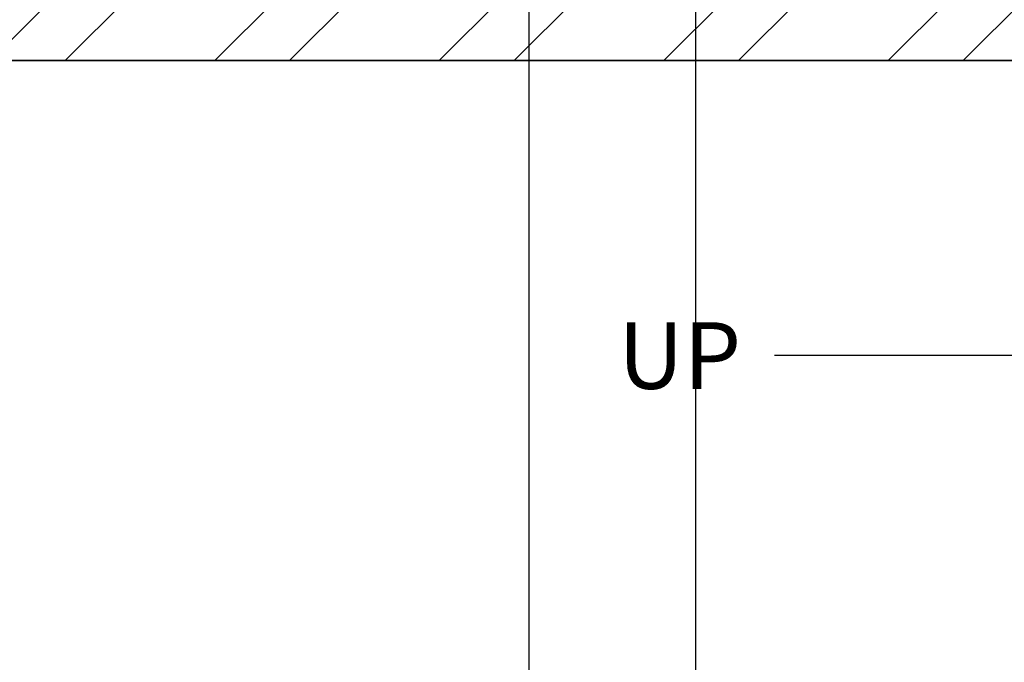
# Model space of a CAD drawing. Units: inches. Extents: x 2166 to 3588, y 1959 to 2628.
# Tile 7 of 13: x 3398 to 3457, y 2067 to 2105. Entities that reach past the tile are written whole.
import ezdxf
from ezdxf import colors
from ezdxf.entities.mleader import LeaderData, LeaderLine
from ezdxf.math import Vec2, Vec3

# ---------------------------------------------------------------- set-up
doc = ezdxf.new("R2010")
doc.units = ezdxf.units.IN
for name, color, linetype, lineweight in [('A-ANNO-DIMS', 2, 'Continuous', 18), ('A-ANNO-SYMB', 136, 'Continuous', 18), ('A-WALL-PATT', 20, 'Continuous', 13), ('WALL', 40, 'Continuous', 35)]:
    doc.layers.add(name, color=color, linetype=linetype, lineweight=lineweight)
doc.styles.get("Standard").update_dxf_attribs({"font": 'arial.ttf'})
doc.dimstyles.get("Standard").update_dxf_attribs({"dimtxt": 0.18, "dimasz": 0.18, "dimexe": 0.18, "dimexo": 0.0625, "dimgap": 0.09, "dimtad": 0, "dimtih": 1, "dimtoh": 1, "dimdec": 4, "dimzin": 0, "dimdsep": 46, "dimtxsty": 'Standard', "dimcen": 0.09, "dimadec": 0, "dimazin": 0, "dimtfac": 1, "dimtdec": 4, "dimtofl": 0, "dimtmove": 0, "dimatfit": 3, "dimfxl": 1, "dimtolj": 1, "dimtzin": 0, "dimarcsym": 0})

# ---------------------------------------------------------------- blocks, each defined once
blk = doc.blocks.new('*D53')
at = {"layer": 'A-ANNO-DIMS', "color": 0, "lineweight": -2, "transparency": 16777216}
for p, q in [((3428.471, 2066.041), (3428.471, 2454.909)), ((3428.651, 2454.729), (3433.26, 2454.729)), ((3438.291, 2454.729), (3433.681, 2454.729)), ((3438.471, 2066.041), (3438.471, 2454.909))]:
    blk.add_line(p, q, dxfattribs=at)
at = {"layer": 'A-ANNO-DIMS', "color": 0, "transparency": 16777216}
for points in [[(3428.651, 2454.759), (3428.651, 2454.699), (3428.471, 2454.729)], [(3438.291, 2454.759), (3438.291, 2454.699), (3438.471, 2454.729)]]:
    blk.add_solid(points, dxfattribs=at)
at = {"layer": 'Defpoints', "color": 0, "transparency": 16777216}
for p in [(3438.471, 2454.729), (3428.471, 2065.979), (3438.471, 2065.979)]:
    blk.add_point(p, dxfattribs=at)
at = {"layer": 'A-ANNO-DIMS', "color": 0, "transparency": 16777216, "insert": (3433.471, 2454.729), "char_height": 0.18, "attachment_point": 5}
blk.add_mtext('\\A1;10', dxfattribs=at)

msp = doc.modelspace()

# ---------------------------------------------------------------- hatches: boundary and pattern name
at = {"layer": 'A-WALL-PATT'}
h = msp.add_hatch(dxfattribs=at)
h.set_pattern_fill('ANSI32', color=256)
h.paths.add_polyline_path([(3563.471, 2429.979), (3227.471, 2429.979), (3227.471, 2021.979), (3563.471, 2021.979)])
h.paths.add_polyline_path([(3236.471, 2420.979), (3554.471, 2420.979), (3554.471, 2111.979), (3236.471, 2111.979)], flags=16)
h.paths.add_polyline_path([(3236.471, 2102.979), (3554.471, 2102.979), (3554.471, 2030.979), (3236.471, 2030.979)], flags=16)
h.paths.add_polyline_path([(3518.471, 2085.283), (3518.471, 2067.979), (3458.471, 2067.979), (3458.471, 2085.283)], flags=0)
h.paths.add_polyline_path([(3434.656, 2082.283), (3442.194, 2082.283), (3442.194, 2087.514), (3434.656, 2087.514)], flags=8)
h.paths.add_polyline_path([(3522.671, 2094.512), (3521.752, 2052.984), (3545.541, 2052.457), (3546.46, 2093.986)], flags=8)

# ---------------------------------------------------------------- linework, layer by layer
at = {"layer": 'WALL'}
msp.add_line((3554.471, 2102.979), (3236.471, 2102.979), dxfattribs=at)

# ---------------------------------------------------------------- dimensions: what is measured, and where the dimension line sits
at = {"layer": 'A-ANNO-DIMS'}
dim = msp.add_linear_dim(base=(3438.471, 2454.729), p1=(3428.471, 2065.979), p2=(3438.471, 2065.979), dimstyle='Standard', override={"dimdec": 0, "dimlfac": 1, "dimrnd": 0, "dimzin": 0, "dimdsep": 46, "dimlunit": 2}, dxfattribs=at)
dim.commit()
dim.dimension.update_dxf_attribs({"geometry": '*D53', "text_midpoint": (3433.471, 2454.729)})

# ---------------------------------------------------------------- leaders
at = {"layer": 'A-ANNO-SYMB'}
ml = msp.add_multileader_mtext('Standard', dxfattribs=at)
ml.set_content('{\\Fsuperos|c0;UP}', color=256)
ml.set_leader_properties()
ml.build(insert=Vec2(0, 0))
ctx = ml.context
ctx.base_point, ctx.plane_origin = Vec3(3433.656, 2085.283), Vec3(3527.576, 2085.283)
ctx.text_align_type = 2
notes = []
notes.append((ctx, [(0, (1, 1, 0), (3451.194, 2085.283), (-1, 0), 8, [(0, [(3527.576, 2085.283)], 0, [])])]))
ctx.mtext.insert, ctx.mtext.alignment, ctx.mtext.flow_direction = Vec3(3441.194, 2087.283), 3, 5
for ctx, leaders in notes:
    for number, flags, end, landing, length, lines in leaders:
        leader = LeaderData()
        leader.index, (leader.has_last_leader_line, leader.has_dogleg_vector, leader.attachment_direction) = number, flags
        leader.last_leader_point, leader.dogleg_vector, leader.dogleg_length = Vec3(end), Vec3(landing), length
        for number, points, colour, breaks in lines:
            line = LeaderLine()
            line.index, line.vertices, line.color, line.breaks = number, Vec3.list(points), colors.encode_raw_color(colour), breaks
            leader.lines.append(line)
        ctx.leaders.append(leader)

doc.saveas('drawing.dxf')
